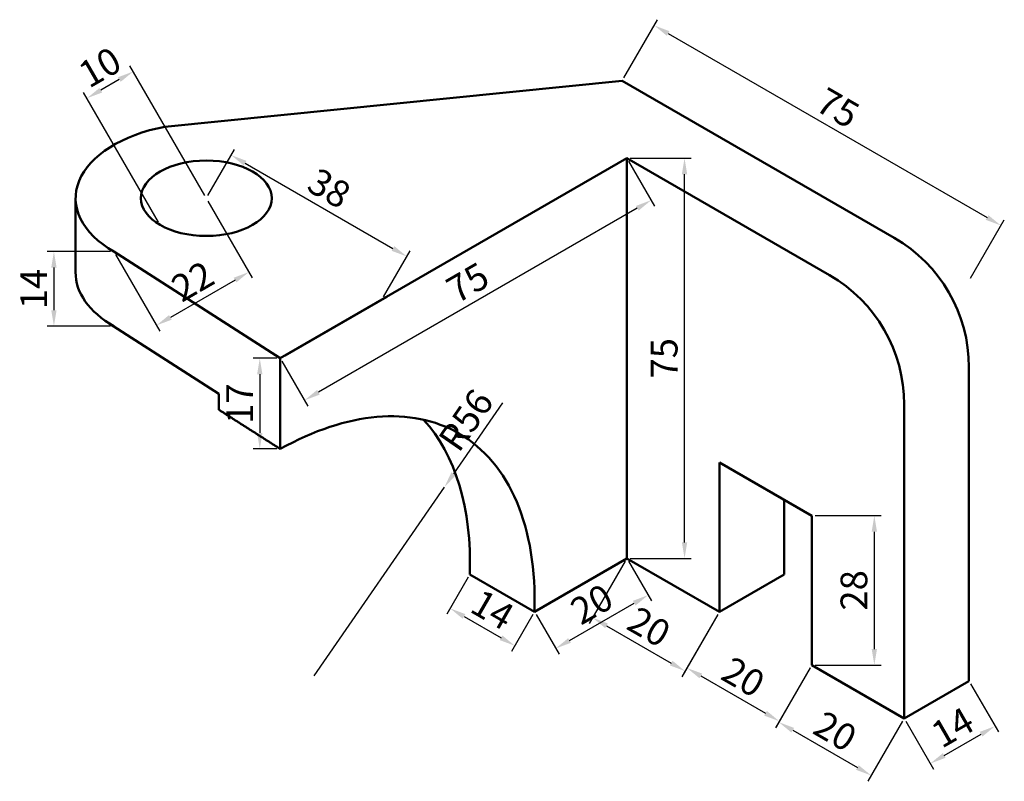
# Model space of a CAD drawing. Units: millimetres. Extents: x -7 to 178, y 5 to 148.
import ezdxf

# ---------------------------------------------------------------- set-up
doc = ezdxf.new("R2010")
doc.units = ezdxf.units.MM
doc.layers.add('M-DIMS', color=2, linetype='Continuous', lineweight=25)
doc.layers.add('M-OUTL', color=7, linetype='Continuous', lineweight=50)
doc.styles.get("Standard").update_dxf_attribs({"font": 'arial.ttf'})
doc.dimstyles.new('ISO-25', dxfattribs={"dimtxt": 5, "dimasz": 3, "dimexe": 1.25, "dimexo": 0.625, "dimtad": 1, "dimtxsty": 'Standard', "dimcen": 2.5, "dimadec": 0, "dimazin": 0, "dimtfac": 1, "dimtmove": 0, "dimatfit": 3, "dimfxl": 1, "dimarcsym": 0})

# ---------------------------------------------------------------- blocks, each defined once
blk = doc.blocks.new('*D1')
at = {"layer": 'Defpoints', "color": 0, "transparency": 16777216}
for p in [(107.24, 121.9), (118.03, 121.9), (107.24, 46.9)]:
    blk.add_point(p, dxfattribs=at)
at = {"layer": 'M-DIMS', "color": 0, "lineweight": -2, "transparency": 16777216}
for p, q in [((107.86, 121.9), (119.28, 121.9)), ((118.03, 49.9), (118.03, 118.9)), ((107.86, 46.9), (119.28, 46.9))]:
    blk.add_line(p, q, dxfattribs=at)
at = {"layer": 'M-DIMS', "color": 0, "transparency": 16777216}
for points in [[(117.53, 118.9), (118.53, 118.9), (118.03, 121.9)], [(117.53, 49.9), (118.53, 49.9), (118.03, 46.9)]]:
    blk.add_solid(points, dxfattribs=at)
at = {"layer": 'M-DIMS', "color": 0, "transparency": 16777216, "insert": (114.86, 84.4), "char_height": 5, "attachment_point": 5, "rotation": 90}
blk.add_mtext('75', dxfattribs=at)
blk = doc.blocks.new('*D2')
at = {"layer": 'Defpoints', "color": 0, "transparency": 16777216}
for p in [(141.88, 54.9), (141.88, 26.9), (153.59, 26.9)]:
    blk.add_point(p, dxfattribs=at)
at = {"layer": 'M-DIMS', "color": 0, "lineweight": -2, "transparency": 16777216}
for p, q in [((142.5, 54.9), (154.84, 54.9)), ((153.59, 51.9), (153.59, 29.9)), ((142.5, 26.9), (154.84, 26.9))]:
    blk.add_line(p, q, dxfattribs=at)
at = {"layer": 'M-DIMS', "color": 0, "transparency": 16777216}
for points in [[(153.09, 51.9), (154.09, 51.9), (153.59, 54.9)], [(153.09, 29.9), (154.09, 29.9), (153.59, 26.9)]]:
    blk.add_solid(points, dxfattribs=at)
at = {"layer": 'M-DIMS', "color": 0, "transparency": 16777216, "insert": (150.41, 40.9), "char_height": 5, "attachment_point": 5, "rotation": 90}
blk.add_mtext('28', dxfattribs=at)
blk = doc.blocks.new('*D3')
at = {"layer": 'Defpoints', "color": 0, "transparency": 16777216}
for p in [(107.24, 46.9), (124.56, 36.9), (118.13, 25.76)]:
    blk.add_point(p, dxfattribs=at)
at = {"layer": 'M-DIMS', "color": 0, "lineweight": -2, "transparency": 16777216}
for p, q in [((106.92, 46.35), (100.18, 34.68)), ((124.24, 36.35), (117.5, 24.68)), ((103.41, 34.26), (115.53, 27.26))]:
    blk.add_line(p, q, dxfattribs=at)
at = {"layer": 'M-DIMS', "color": 0, "transparency": 16777216}
for points in [[(103.66, 34.7), (103.16, 33.83), (100.81, 35.76)], [(115.78, 27.7), (115.28, 26.83), (118.13, 25.76)]]:
    blk.add_solid(points, dxfattribs=at)
at = {"layer": 'M-DIMS', "color": 0, "transparency": 16777216, "insert": (111.06, 33.51), "char_height": 5, "attachment_point": 5, "rotation": 330}
blk.add_mtext('20', dxfattribs=at)
blk = doc.blocks.new('*D4')
at = {"layer": 'Defpoints', "color": 0, "transparency": 16777216}
for p in [(124.56, 36.9), (141.88, 26.9), (135.8, 16.36)]:
    blk.add_point(p, dxfattribs=at)
at = {"layer": 'M-DIMS', "color": 0, "lineweight": -2, "transparency": 16777216}
for p, q in [((124.24, 36.35), (117.85, 25.28)), ((141.56, 26.35), (135.17, 15.28)), ((121.07, 24.86), (133.2, 17.86))]:
    blk.add_line(p, q, dxfattribs=at)
at = {"layer": 'M-DIMS', "color": 0, "transparency": 16777216}
for points in [[(121.32, 25.3), (120.82, 24.43), (118.48, 26.36)], [(133.45, 18.3), (132.95, 17.43), (135.8, 16.36)]]:
    blk.add_solid(points, dxfattribs=at)
at = {"layer": 'M-DIMS', "color": 0, "transparency": 16777216, "insert": (128.72, 24.11), "char_height": 5, "attachment_point": 5, "rotation": 330}
blk.add_mtext('20', dxfattribs=at)
blk = doc.blocks.new('*D5')
at = {"layer": 'Defpoints', "color": 0, "transparency": 16777216}
for p in [(141.88, 26.9), (159.2, 16.9), (153.02, 6.19)]:
    blk.add_point(p, dxfattribs=at)
at = {"layer": 'M-DIMS', "color": 0, "lineweight": -2, "transparency": 16777216}
for p, q in [((141.56, 26.35), (135.07, 15.11)), ((158.89, 16.35), (152.39, 5.11)), ((138.29, 14.69), (150.42, 7.69))]:
    blk.add_line(p, q, dxfattribs=at)
at = {"layer": 'M-DIMS', "color": 0, "transparency": 16777216}
for points in [[(138.54, 15.12), (138.04, 14.26), (135.7, 16.19)], [(150.67, 8.12), (150.17, 7.26), (153.02, 6.19)]]:
    blk.add_solid(points, dxfattribs=at)
at = {"layer": 'M-DIMS', "color": 0, "transparency": 16777216, "insert": (145.95, 13.94), "char_height": 5, "attachment_point": 5, "rotation": 330}
blk.add_mtext('20', dxfattribs=at)
blk = doc.blocks.new('*D6')
at = {"layer": 'Defpoints', "color": 0, "transparency": 16777216}
for p in [(106.37, 136.4), (177.32, 109.28), (171.32, 98.9)]:
    blk.add_point(p, dxfattribs=at)
at = {"layer": 'M-DIMS', "color": 0, "lineweight": -2, "transparency": 16777216}
for p, q in [((106.68, 136.94), (112.99, 147.86)), ((114.96, 145.28), (174.72, 110.78)), ((171.63, 99.44), (177.94, 110.36))]:
    blk.add_line(p, q, dxfattribs=at)
at = {"layer": 'M-DIMS', "color": 0, "transparency": 16777216}
for points in [[(115.21, 145.71), (114.71, 144.85), (112.37, 146.78)], [(174.97, 111.21), (174.47, 110.35), (177.32, 109.28)]]:
    blk.add_solid(points, dxfattribs=at)
at = {"layer": 'M-DIMS', "color": 0, "transparency": 16777216, "insert": (146.43, 130.78), "char_height": 5, "attachment_point": 5, "rotation": 330}
blk.add_mtext('75', dxfattribs=at)
blk = doc.blocks.new('*D7')
at = {"layer": 'Defpoints', "color": 0, "transparency": 16777216}
for p in [(73.05, 60.27), (48.65, 24.89)]:
    blk.add_point(p, dxfattribs=at)
at = {"layer": 'M-DIMS', "color": 0, "lineweight": -2, "transparency": 16777216}
for p, q in [((83.95, 76.07), (74.76, 62.74)), ((48.65, 24.89), (73.05, 60.27))]:
    blk.add_line(p, q, dxfattribs=at)
at = {"layer": 'M-DIMS', "color": 0, "transparency": 16777216}
blk.add_solid([(74.34, 63.02), (75.17, 62.45), (73.05, 60.27)], dxfattribs=at)
at = {"layer": 'M-DIMS', "color": 0, "transparency": 16777216, "insert": (77.59, 72.44), "char_height": 5, "attachment_point": 5, "rotation": 55.4006}
blk.add_mtext('R56', dxfattribs=at)
blk = doc.blocks.new('*D8')
at = {"layer": 'Defpoints', "color": 0, "transparency": 16777216}
for p in [(42.28, 84.4), (38.44, 67.4), (42.28, 67.4)]:
    blk.add_point(p, dxfattribs=at)
at = {"layer": 'M-DIMS', "color": 0, "lineweight": -2, "transparency": 16777216}
for p, q in [((41.66, 84.4), (37.19, 84.4)), ((38.44, 81.4), (38.44, 70.4)), ((41.66, 67.4), (37.19, 67.4))]:
    blk.add_line(p, q, dxfattribs=at)
at = {"layer": 'M-DIMS', "color": 0, "transparency": 16777216}
for points in [[(37.94, 81.4), (38.94, 81.4), (38.44, 84.4)], [(37.94, 70.4), (38.94, 70.4), (38.44, 67.4)]]:
    blk.add_solid(points, dxfattribs=at)
at = {"layer": 'M-DIMS', "color": 0, "transparency": 16777216, "insert": (35.31, 75.9), "char_height": 5, "attachment_point": 5, "rotation": 90}
blk.add_mtext('17', dxfattribs=at)
blk = doc.blocks.new('*D9')
at = {"layer": 'Defpoints', "color": 0, "transparency": 16777216}
for p in [(77.79, 43.9), (89.92, 36.9), (86.23, 30.52)]:
    blk.add_point(p, dxfattribs=at)
at = {"layer": 'M-DIMS', "color": 0, "lineweight": -2, "transparency": 16777216}
for p, q in [((77.48, 43.35), (73.48, 36.44)), ((76.71, 36.02), (83.64, 32.02)), ((89.6, 36.35), (85.61, 29.44))]:
    blk.add_line(p, q, dxfattribs=at)
at = {"layer": 'M-DIMS', "color": 0, "transparency": 16777216}
for points in [[(76.96, 36.45), (76.46, 35.58), (74.11, 37.52)], [(83.89, 32.45), (83.39, 31.58), (86.23, 30.52)]]:
    blk.add_solid(points, dxfattribs=at)
at = {"layer": 'M-DIMS', "color": 0, "transparency": 16777216, "insert": (81.74, 36.73), "char_height": 5, "attachment_point": 5, "rotation": 330}
blk.add_mtext('14', dxfattribs=at)
blk = doc.blocks.new('*D10')
at = {"layer": 'Defpoints', "color": 0, "transparency": 16777216}
for p in [(171.32, 23.9), (159.2, 16.9), (176.2, 15.44)]:
    blk.add_point(p, dxfattribs=at)
at = {"layer": 'M-DIMS', "color": 0, "lineweight": -2, "transparency": 16777216}
for p, q in [((171.63, 23.35), (176.83, 14.36)), ((159.51, 16.35), (164.7, 7.36)), ((166.68, 9.94), (173.6, 13.94))]:
    blk.add_line(p, q, dxfattribs=at)
at = {"layer": 'M-DIMS', "color": 0, "transparency": 16777216}
for points in [[(173.35, 14.38), (173.85, 13.51), (176.2, 15.44)], [(166.43, 10.38), (166.93, 9.51), (164.08, 8.44)]]:
    blk.add_solid(points, dxfattribs=at)
at = {"layer": 'M-DIMS', "color": 0, "transparency": 16777216, "insert": (168.57, 14.66), "char_height": 5, "attachment_point": 5, "rotation": 30}
blk.add_mtext('14', dxfattribs=at)
blk = doc.blocks.new('*D11')
at = {"layer": 'Defpoints', "color": 0, "transparency": 16777216}
for p in [(11.11, 104.4), (-0.13, 90.4), (11.11, 90.4)]:
    blk.add_point(p, dxfattribs=at)
at = {"layer": 'M-DIMS', "color": 0, "lineweight": -2, "transparency": 16777216}
for p, q in [((10.48, 104.4), (-1.38, 104.4)), ((-0.13, 101.4), (-0.13, 93.4)), ((10.48, 90.4), (-1.38, 90.4))]:
    blk.add_line(p, q, dxfattribs=at)
at = {"layer": 'M-DIMS', "color": 0, "transparency": 16777216}
for points in [[(-0.63, 101.4), (0.37, 101.4), (-0.13, 104.4)], [(-0.63, 93.4), (0.37, 93.4), (-0.13, 90.4)]]:
    blk.add_solid(points, dxfattribs=at)
at = {"layer": 'M-DIMS', "color": 0, "transparency": 16777216, "insert": (-3.26, 97.4), "char_height": 5, "attachment_point": 5, "rotation": 90}
blk.add_mtext('14', dxfattribs=at)
blk = doc.blocks.new('*D12')
at = {"layer": 'Defpoints', "color": 0, "transparency": 16777216}
for p in [(6.06, 133.14), (28.43, 114.4), (19.77, 109.4)]:
    blk.add_point(p, dxfattribs=at)
at = {"layer": 'M-DIMS', "color": 0, "lineweight": -2, "transparency": 16777216}
for p, q in [((28.12, 114.94), (14.09, 139.22)), ((12.12, 136.64), (8.66, 134.64)), ((19.45, 109.94), (5.43, 134.22))]:
    blk.add_line(p, q, dxfattribs=at)
at = {"layer": 'M-DIMS', "color": 0, "transparency": 16777216}
for points in [[(11.87, 137.07), (12.37, 136.21), (14.72, 138.14)], [(8.41, 135.07), (8.91, 134.21), (6.06, 133.14)]]:
    blk.add_solid(points, dxfattribs=at)
at = {"layer": 'M-DIMS', "color": 0, "transparency": 16777216, "insert": (8.8, 138.39), "char_height": 5, "attachment_point": 5, "rotation": 30}
blk.add_mtext('10', dxfattribs=at)
blk = doc.blocks.new('*D13')
at = {"layer": 'Defpoints', "color": 0, "transparency": 16777216}
for p in [(28.43, 114.4), (66, 103.48), (61.34, 95.4)]:
    blk.add_point(p, dxfattribs=at)
at = {"layer": 'M-DIMS', "color": 0, "lineweight": -2, "transparency": 16777216}
for p, q in [((28.74, 114.94), (33.72, 123.56)), ((35.69, 120.98), (63.4, 104.98)), ((61.65, 95.94), (66.63, 104.56))]:
    blk.add_line(p, q, dxfattribs=at)
at = {"layer": 'M-DIMS', "color": 0, "transparency": 16777216}
for points in [[(35.94, 121.41), (35.44, 120.54), (33.09, 122.48)], [(63.65, 105.41), (63.15, 104.54), (66, 103.48)]]:
    blk.add_solid(points, dxfattribs=at)
at = {"layer": 'M-DIMS', "color": 0, "transparency": 16777216, "insert": (51.14, 115.73), "char_height": 5, "attachment_point": 5, "rotation": 330}
blk.add_mtext('38', dxfattribs=at)
blk = doc.blocks.new('*D14')
at = {"layer": 'Defpoints', "color": 0, "transparency": 16777216}
for p in [(107.24, 121.9), (42.28, 84.4), (46.83, 76.53)]:
    blk.add_point(p, dxfattribs=at)
at = {"layer": 'M-DIMS', "color": 0, "lineweight": -2, "transparency": 16777216}
for p, q in [((107.55, 121.35), (112.4, 112.94)), ((109.18, 112.53), (49.43, 78.03)), ((42.6, 83.85), (47.45, 75.44))]:
    blk.add_line(p, q, dxfattribs=at)
at = {"layer": 'M-DIMS', "color": 0, "transparency": 16777216}
for points in [[(108.93, 112.96), (109.43, 112.09), (111.78, 114.03)], [(49.18, 78.46), (49.68, 77.59), (46.83, 76.53)]]:
    blk.add_solid(points, dxfattribs=at)
at = {"layer": 'M-DIMS', "color": 0, "transparency": 16777216, "insert": (77.72, 98.02), "char_height": 5, "attachment_point": 5, "rotation": 30}
blk.add_mtext('75', dxfattribs=at)
blk = doc.blocks.new('*D15')
at = {"layer": 'Defpoints', "color": 0, "transparency": 16777216}
for p in [(28.43, 114.4), (11.11, 104.4), (19.09, 90.57)]:
    blk.add_point(p, dxfattribs=at)
at = {"layer": 'M-DIMS', "color": 0, "lineweight": -2, "transparency": 16777216}
for p, q in [((28.74, 113.85), (37.04, 99.48)), ((11.42, 103.85), (19.72, 89.48)), ((33.81, 99.07), (21.69, 92.07))]:
    blk.add_line(p, q, dxfattribs=at)
at = {"layer": 'M-DIMS', "color": 0, "transparency": 16777216}
for points in [[(33.56, 99.5), (34.06, 98.63), (36.41, 100.57)], [(21.44, 92.5), (21.94, 91.63), (19.09, 90.57)]]:
    blk.add_solid(points, dxfattribs=at)
at = {"layer": 'M-DIMS', "color": 0, "transparency": 16777216, "insert": (26.18, 98.28), "char_height": 5, "attachment_point": 5, "rotation": 30}
blk.add_mtext('22', dxfattribs=at)
blk = doc.blocks.new('*D16')
at = {"layer": 'Defpoints', "color": 0, "transparency": 16777216}
for p in [(107.24, 46.9), (111.21, 40.01), (89.92, 36.9)]:
    blk.add_point(p, dxfattribs=at)
at = {"layer": 'M-DIMS', "color": 0, "lineweight": -2, "transparency": 16777216}
for p, q in [((107.55, 46.35), (111.84, 38.93)), ((96.49, 31.51), (108.61, 38.51)), ((90.23, 36.35), (94.52, 28.93))]:
    blk.add_line(p, q, dxfattribs=at)
at = {"layer": 'M-DIMS', "color": 0, "transparency": 16777216}
for points in [[(108.36, 38.94), (108.86, 38.07), (111.21, 40.01)], [(96.24, 31.94), (96.74, 31.07), (93.89, 30.01)]]:
    blk.add_solid(points, dxfattribs=at)
at = {"layer": 'M-DIMS', "color": 0, "transparency": 16777216, "insert": (100.96, 37.76), "char_height": 5, "attachment_point": 5, "rotation": 30}
blk.add_mtext('20', dxfattribs=at)

msp = doc.modelspace()

# ---------------------------------------------------------------- linework, layer by layer
at = {"layer": 'M-OUTL'}
for p, q in [((106.37, 136.395), (20.682, 127.812)), ((157.322, 106.978), (106.37, 136.395)), ((107.236, 121.895), (42.284, 84.395)), ((107.236, 46.895), (107.236, 121.895)), ((107.236, 121.895), (145.198, 99.978)), ((3.934, 100.254), (3.934, 114.254)), ((42.284, 84.395), (11.107, 104.395)), ((43.209, 84.929), (62.261, 95.929)), ((10.233, 90.928), (30.79, 77.759)), ((42.284, 84.395), (42.284, 67.395)), ((171.322, 23.895), (171.322, 82.73)), ((30.79, 74.742), (30.79, 77.759)), ((159.198, 16.895), (159.198, 75.73)), ((124.557, 36.895), (124.557, 64.895)), ((124.557, 64.895), (141.877, 54.895)), ((136.681, 43.895), (136.681, 57.895)), ((141.877, 54.895), (141.877, 26.895)), ((89.916, 36.895), (107.236, 46.895)), ((107.236, 46.895), (124.557, 36.895)), ((89.916, 36.895), (77.791, 43.895)), ((124.557, 36.895), (136.681, 43.895)), ((141.877, 26.895), (159.198, 16.895)), ((141.877, 26.895), (159.198, 16.895)), ((159.198, 16.895), (171.322, 23.895))]:
    msp.add_line(p, q, dxfattribs=at)
msp.add_lwpolyline([(42.284, 67.395), (42.164, 67.472), (42.045, 67.548), (41.925, 67.625), (41.805, 67.702), (41.685, 67.778), (41.566, 67.855), (41.446, 67.931), (41.326, 68.008), (41.206, 68.085), (41.087, 68.161), (40.967, 68.238), (40.847, 68.314), (40.727, 68.391), (40.608, 68.467), (40.488, 68.544), (40.368, 68.62), (40.248, 68.697), (40.129, 68.774), (40.009, 68.85), (39.889, 68.927), (39.769, 69.003), (39.65, 69.08), (39.53, 69.156), (39.41, 69.233), (39.29, 69.31), (39.171, 69.386), (39.051, 69.463), (38.931, 69.539), (38.811, 69.616), (38.692, 69.692), (38.572, 69.769), (38.452, 69.845), (38.333, 69.922), (38.213, 69.998), (38.093, 70.075), (37.973, 70.152), (37.854, 70.228), (37.734, 70.305), (37.614, 70.381), (37.494, 70.458), (37.375, 70.534), (37.255, 70.611), (37.135, 70.687), (37.015, 70.764), (36.896, 70.84), (36.776, 70.917), (36.656, 70.993), (36.536, 71.07), (36.417, 71.146), (36.297, 71.223), (36.177, 71.299), (36.057, 71.376), (35.938, 71.453), (35.818, 71.529), (35.698, 71.606), (35.579, 71.682), (35.459, 71.759), (35.339, 71.835), (35.219, 71.912), (35.1, 71.988), (34.98, 72.065), (34.86, 72.141), (34.74, 72.218), (34.621, 72.294), (34.501, 72.371), (34.381, 72.447), (34.261, 72.524), (34.142, 72.6), (34.022, 72.677), (33.902, 72.753), (33.783, 72.83), (33.663, 72.906), (33.543, 72.983), (33.423, 73.059), (33.304, 73.136), (33.184, 73.212), (33.064, 73.289), (32.945, 73.365), (32.825, 73.442), (32.705, 73.518), (32.585, 73.595), (32.466, 73.671), (32.346, 73.748), (32.226, 73.824), (32.106, 73.9), (31.987, 73.977), (31.867, 74.053), (31.747, 74.13), (31.628, 74.206), (31.508, 74.283), (31.388, 74.359), (31.268, 74.436), (31.149, 74.512), (31.029, 74.589), (30.909, 74.665), (30.79, 74.742)], dxfattribs=at)
for centre in [(143.322, 82.73), (131.198, 75.73)]:
    msp.add_arc(centre, 28, 0, 60, dxfattribs=at)
for centre, major_axis, start_param, end_param in [((28.428, 114.395), (-24.495, 0), 5.0341395, 7.0685835), ((28.428, 100.395), (-24.495, 0), 6.2731846, 7.0685835), ((41.449, 10.922), (-34.293, -59.397), 3.1415927, 3.9097766), ((29.325, 17.922), (-34.293, -59.397), 2.3203238, 2.963882), ((41.449, 10.922), (-34.293, -59.397), 2.3203238, 3.1415927)]:
    msp.add_ellipse(centre, major_axis=major_axis, ratio=0.5773503, start_param=start_param, end_param=end_param, dxfattribs=at)
msp.add_ellipse((28.428, 114.395), major_axis=(-12.247, 0), ratio=0.5773503, dxfattribs=at)

# ---------------------------------------------------------------- dimensions: what is measured, and where the dimension line sits
at = {"layer": 'M-DIMS'}
for p1, p2, distance, picture, middle in [((106.37, 136.395), (171.322, 98.895), 11.993, '*D6', (146.427, 130.775)), ((28.428, 114.395), (19.767, 109.395), -27.417, '*D12', (8.8, 138.391)), ((28.428, 114.395), (61.337, 95.395), 9.332, '*D13', (51.138, 115.731)), ((107.236, 121.895), (42.284, 84.395), 9.087, '*D14', (77.72, 98.019)), ((89.916, 36.895), (107.236, 46.895), -7.953, '*D16', (100.963, 37.76)), ((107.236, 46.895), (124.557, 36.895), -12.855, '*D3', (111.058, 33.515)), ((77.791, 43.895), (89.916, 36.895), -7.364, '*D9', (81.739, 36.733)), ((124.557, 36.895), (141.877, 26.895), -12.162, '*D4', (128.725, 24.115)), ((141.877, 26.895), (159.198, 16.895), -12.362, '*D5', (145.945, 13.942)), ((159.198, 16.895), (171.322, 23.895), -9.759, '*D10', (168.572, 14.659))]:
    dim = msp.add_aligned_dim(p1=p1, p2=p2, distance=distance, dimstyle='ISO-25', override={"dimclrd": 0, "dimclre": 0, "dimclrt": 0}, dxfattribs=at)
    dim.commit()
    dim.dimension.update_dxf_attribs({"geometry": picture, "text_midpoint": middle})
for base, p1, p2, picture, middle in [((118.032, 121.895), (107.236, 46.895), (107.236, 121.895), '*D1', (114.864, 84.395)), ((-0.127, 90.395), (11.107, 104.395), (11.107, 90.395), '*D11', (-3.262, 97.395)), ((38.443, 67.395), (42.284, 84.395), (42.284, 67.395), '*D8', (35.307, 75.895)), ((153.593, 26.895), (141.877, 54.895), (141.877, 26.895), '*D2', (150.415, 40.895))]:
    dim = msp.add_linear_dim(base=base, p1=p1, p2=p2, angle=90, dimstyle='ISO-25', override={"dimclrd": 0, "dimclre": 0, "dimclrt": 0}, dxfattribs=at)
    dim.commit()
    dim.dimension.update_dxf_attribs({"geometry": picture, "text_midpoint": middle})
dim = msp.add_aligned_dim(p1=(28.428, 114.395), p2=(11.107, 104.395), distance=15.968, text='22', dimstyle='ISO-25', override={"dimclrd": 0, "dimclre": 0, "dimclrt": 0}, dxfattribs=at)
dim.commit()
dim.dimension.update_dxf_attribs({"geometry": '*D15', "text_midpoint": (26.184, 98.282)})
dim = msp.add_radius_dim(center=(48.647, 24.889), mpoint=(73.052, 60.268), text='R56', dimstyle='ISO-25', override={"dimclrd": 0, "dimclre": 0, "dimclrt": 0}, dxfattribs=at)
dim.commit()
dim.dimension.update_dxf_attribs({"geometry": '*D7', "text_midpoint": (77.589, 72.441)})

doc.saveas('drawing.dxf')
